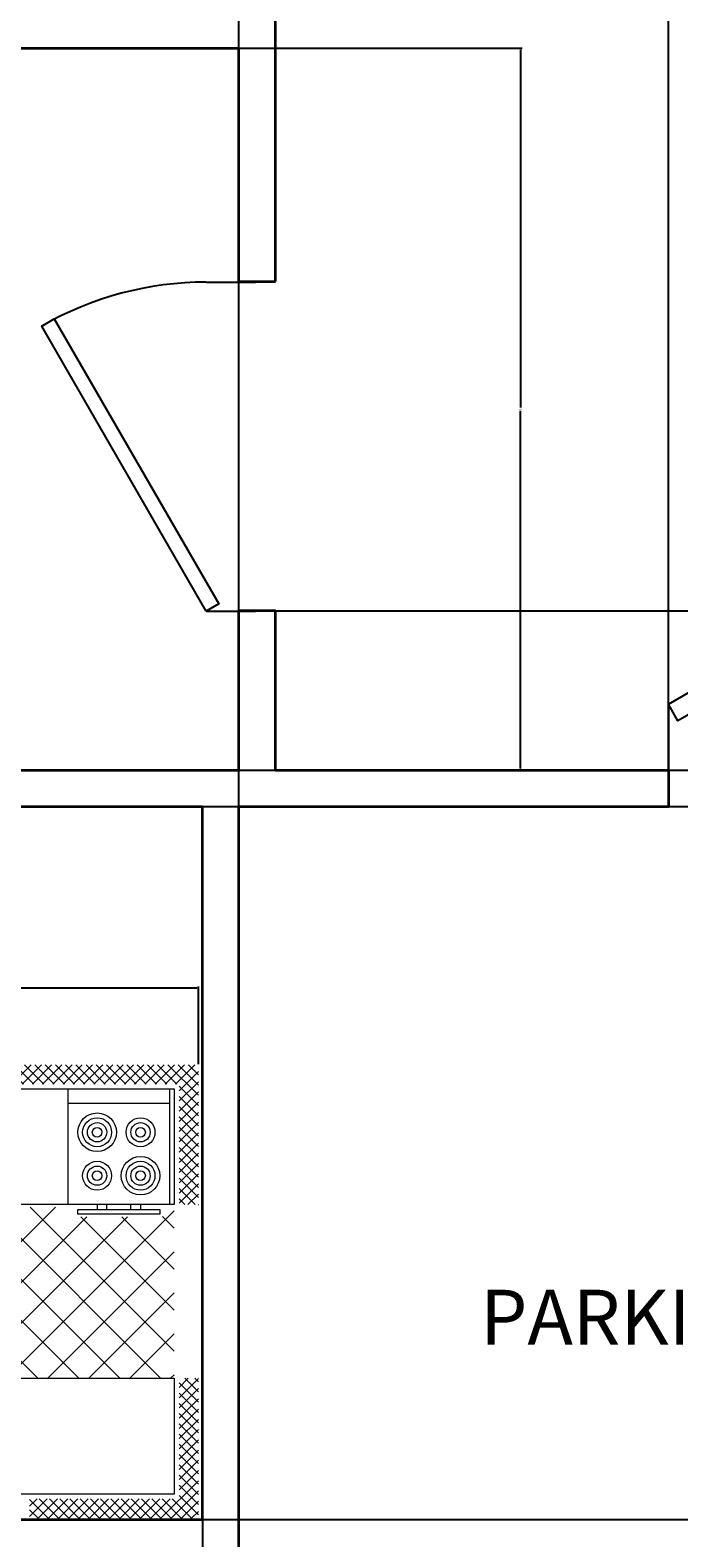
# Model space of a CAD drawing. Units: feet. Extents: x 3746 to 4170, y 1475 to 2148.
# Tile 3 of 5: x 3884 to 3955, y 1755 to 1920. Entities that reach past the tile are written whole.
import ezdxf

# ---------------------------------------------------------------- set-up
doc = ezdxf.new("R2010")
doc.units = ezdxf.units.FT
for name, color, linetype, lineweight in [('A-ANNO-DIMS', 2, 'Continuous', 18), ('A-AREA-IDEN', 7, 'Continuous', 25), ('A-FLOR-FIXT', 9, 'Continuous', 18), ('DOOR', 135, 'Continuous', 25), ('INWER WALL', 30, 'Continuous', 35)]:
    doc.layers.add(name, color=color, linetype=linetype, lineweight=lineweight)
doc.styles.get("Standard").update_dxf_attribs({"font": 'arial.ttf'})
doc.dimstyles.get("Standard").update_dxf_attribs({"dimtxt": 0.18, "dimasz": 0.18, "dimexe": 0.18, "dimexo": 0.0625, "dimgap": 0.09, "dimtad": 0, "dimtih": 1, "dimtoh": 1, "dimdec": 4, "dimzin": 0, "dimdsep": 46, "dimtxsty": 'Standard', "dimcen": 0.09, "dimadec": 0, "dimazin": 0, "dimtfac": 1, "dimtdec": 4, "dimtofl": 0, "dimtmove": 0, "dimatfit": 3, "dimfxl": 1, "dimtolj": 1, "dimtzin": 0, "dimarcsym": 0})

# ---------------------------------------------------------------- blocks, each defined once
blk = doc.blocks.new('*U2')
for p, q in [((0, 0), (0, -6)), ((40, 0), (40, -6))]:
    blk.add_line(p, q)
blk.add_lwpolyline([(0, 0), (34.64, 20), (35.52, 18.48), (0.87, -1.52)], close=True)
blk.add_arc((0, 0), 40, 0, 30)
blk = doc.blocks.new('Kitchen Layout - 7 x 8 ft')
for p, q in [((-5, 81.32), (2.68, 89)), ((-5, 83.44), (0.56, 89)), ((-5, 85.56), (-1.56, 89)), ((-5, 87.68), (-3.68, 89)), ((-1, 84.97), (-5, 88.97)), ((1.09, 85), (-2.91, 89)), ((3.21, 85), (-0.79, 89)), ((0.81, 85), (4.81, 89)), ((5.34, 85), (1.34, 89)), ((2.93, 85), (6.93, 89)), ((7.46, 85), (3.46, 89)), ((5.05, 85), (9.05, 89)), ((9.58, 85), (5.58, 89)), ((7.17, 85), (11.17, 89)), ((11.7, 85), (7.7, 89)), ((9.29, 85), (13.29, 89)), ((13.82, 85), (9.82, 89)), ((11.41, 85), (15.41, 89)), ((15.94, 85), (11.94, 89)), ((13.53, 85), (17.53, 89)), ((18.06, 85), (14.06, 89)), ((15.65, 85), (19.65, 89)), ((20.18, 85), (16.18, 89)), ((17.78, 85), (21.78, 89)), ((22.31, 85), (18.31, 89)), ((19.9, 85), (23.9, 89)), ((24.43, 85), (20.43, 89)), ((22.02, 85), (26.02, 89)), ((26.55, 85), (22.55, 89)), ((24.14, 85), (28.14, 89)), ((28.67, 85), (24.67, 89)), ((26.26, 85), (30.26, 89)), ((30.79, 85), (26.79, 89)), ((28.38, 85), (32.38, 89)), ((32.91, 85), (28.91, 89)), ((30.5, 85), (34.5, 89)), ((35.03, 85), (31.03, 89)), ((32.63, 85), (36.63, 89)), ((37.16, 85), (33.16, 89)), ((34.75, 85), (38.75, 89)), ((39.28, 85), (35.28, 89)), ((36.87, 85), (40.87, 89)), ((41.4, 85), (37.4, 89)), ((38.99, 85), (42.99, 89)), ((43.52, 85), (39.52, 89)), ((41.11, 85), (45.11, 89)), ((45.64, 85), (41.64, 89)), ((43.23, 85), (47.23, 89)), ((47.76, 85), (43.76, 89)), ((45.35, 85), (49.35, 89)), ((49.88, 85), (45.88, 89)), ((47.47, 85), (51.47, 89)), ((52, 85), (48, 89)), ((49.6, 85), (53.6, 89)), ((54.13, 85), (50.13, 89)), ((51.72, 85), (55.72, 89)), ((56.25, 85), (52.25, 89)), ((53.84, 85), (57.84, 89)), ((58.37, 85), (54.37, 89)), ((55.96, 85), (59.96, 89)), ((60.49, 85), (56.49, 89)), ((58.08, 85), (62.08, 89)), ((62.61, 85), (58.61, 89)), ((60.2, 85), (64.2, 89)), ((64.73, 85), (60.73, 89)), ((62.32, 85), (66.32, 89)), ((66.85, 85), (62.85, 89)), ((64.45, 85), (68.45, 89)), ((68.97, 85), (64.97, 89)), ((66.57, 85), (70.57, 89)), ((71.1, 85), (67.1, 89)), ((68.69, 85), (72.69, 89)), ((73.22, 85), (69.22, 89)), ((70.81, 85), (74.81, 89)), ((75.34, 85), (71.34, 89)), ((72.93, 85), (76.93, 89)), ((77.46, 85), (73.46, 89)), ((75.05, 85), (79.05, 89)), ((79.58, 85), (75.58, 89)), ((77.17, 85), (81.17, 89)), ((81.7, 85), (77.7, 89)), ((79.29, 85), (83.29, 89)), ((83.82, 85), (79.82, 89)), ((81.42, 85), (85.42, 89)), ((85.95, 85), (81.95, 89)), ((83.54, 85), (87.54, 89)), ((88.07, 85), (84.07, 89)), ((85.66, 85), (89.66, 89)), ((90.19, 85), (86.19, 89)), ((87.78, 85), (91.78, 89)), ((92.31, 85), (88.31, 89)), ((89.9, 85), (93.9, 89)), ((94.43, 85), (90.43, 89)), ((92.02, 85), (96.02, 89)), ((96.55, 85), (92.55, 89)), ((94.14, 85), (98.14, 89)), ((101, 82.67), (94.67, 89)), ((96.27, 85), (100.27, 89)), ((101, 84.79), (96.79, 89)), ((97, 83.61), (101, 87.61)), ((101, 86.92), (98.92, 89)), ((-1, 82.85), (-5, 86.85)), ((-1, 80.73), (-5, 84.73)), ((97, 81.49), (101, 85.49)), ((101, 80.55), (97, 84.55)), ((-5, 79.19), (-1, 83.19)), ((-1, 78.61), (-5, 82.61)), ((34, 84), (96, 84)), ((34, 60), (34, 84)), ((96, 84), (96, 60)), ((97, 79.37), (101, 83.37)), ((101, 78.43), (97, 82.43)), ((-5, 77.07), (-1, 81.07)), ((-1, 76.49), (-5, 80.49)), ((-5, 74.95), (-1, 78.95)), ((-1, 74.36), (-5, 78.36)), ((74, 81), (95, 81)), ((97, 77.25), (101, 81.25)), ((101, 76.31), (97, 80.31)), ((97, 75.13), (101, 79.13)), ((101, 74.19), (97, 78.19)), ((-5, 72.83), (-1, 76.83)), ((-1, 72.24), (-5, 76.24)), ((97, 73.01), (101, 77.01)), ((101, 72.07), (97, 76.07)), ((-5, 70.71), (-1, 74.71)), ((-1, 70.12), (-5, 74.12)), ((-5, 68.59), (-1, 72.59)), ((-1, 68), (-5, 72)), ((97, 70.89), (101, 74.89)), ((101, 69.95), (97, 73.95)), ((97, 68.76), (101, 72.76)), ((-5, 66.47), (-1, 70.47)), ((-1, 65.88), (-5, 69.88)), ((101, 67.82), (97, 71.82)), ((97, 66.64), (101, 70.64)), ((101, 65.7), (97, 69.7)), ((-5, 64.35), (-1, 68.35)), ((-1, 63.76), (-5, 67.76)), ((-5, 62.22), (-1, 66.22)), ((-1, 61.64), (-5, 65.64)), ((97, 64.52), (101, 68.52)), ((101, 63.58), (97, 67.58)), ((97, 62.4), (101, 66.4)), ((-5, 60.1), (-1, 64.1)), ((-1, 59.52), (-5, 63.52)), ((101, 61.46), (97, 65.46)), ((97, 60.28), (101, 64.28)), ((100.34, 60), (97, 63.34)), ((-5, 57.98), (-1, 61.98)), ((-1, 57.39), (-5, 61.39)), ((-4.86, 56), (-1, 59.86)), ((10.4, 24), (45.9, 59.5)), ((18.88, 24), (54.38, 59.5)), ((27.37, 24), (62.87, 59.5)), ((33.03, 55.11), (37.41, 59.5)), ((96, 60), (34, 60)), ((35.85, 24), (71.35, 59.5)), ((76.2, 24), (40.7, 59.5)), ((84.68, 24), (49.18, 59.5)), ((93.17, 24), (57.67, 59.5)), ((96, 29.65), (66.15, 59.5)), ((80, 60), (80, 59)), ((82, 59), (82, 60)), ((87, 59), (87, 60)), ((89, 60), (89, 59)), ((98.22, 60), (97, 61.22)), ((98.84, 60), (101, 62.16)), ((100.96, 60), (101, 60.04)), ((-1.73, 56), (-5, 59.27)), ((-3.85, 56), (-5, 57.15)), ((-2.74, 56), (-1, 57.74)), ((0, 57), (33, 57)), ((67.71, 24), (33.68, 58.04)), ((44.34, 24), (77.84, 57.5)), ((52.82, 24), (86.32, 57.5)), ((61.31, 24), (96, 58.69)), ((96, 38.14), (76.64, 57.5)), ((96, 46.63), (85.13, 57.5)), ((96, 55.11), (93.57, 57.54)), ((0, 30.57), (24.43, 55)), ((0, 39.06), (15.94, 55)), ((0, 47.54), (7.46, 55)), ((1.91, 24), (32.91, 55)), ((33.77, 24), (2.77, 55)), ((42.26, 24), (11.26, 55)), ((50.74, 24), (19.74, 55)), ((59.23, 24), (28.23, 55)), ((31, 55), (31, 56)), ((32, 55), (31, 55)), ((32, 56), (32, 55)), ((69.79, 24), (96, 50.21)), ((25.29, 24), (0, 49.29)), ((16.8, 24), (0, 40.8)), ((78.28, 24), (96, 41.72)), ((8.32, 24), (0, 32.32)), ((86.76, 24), (96, 33.24)), ((-5, 21.92), (-2.92, 24)), ((-5, 19.8), (-1, 23.8)), ((-1, 19.21), (-5, 23.21)), ((-1, 21.33), (-3.67, 24)), ((-1, 23.45), (-1.55, 24)), ((0, 24), (96, 24)), ((0, 0), (0, 24)), ((95.25, 24), (96, 24.75)), ((96, 24), (96, 0)), ((97, 22.1), (98.9, 24)), ((97, 19.97), (101, 23.97)), ((101, 19.03), (97, 23.03)), ((101, 21.16), (98.16, 24)), ((101, 23.28), (100.28, 24)), ((-5, 17.68), (-1, 21.68)), ((-1, 17.09), (-5, 21.09)), ((-5, 15.55), (-1, 19.55)), ((-1, 14.97), (-5, 18.97)), ((97, 17.85), (101, 21.85)), ((101, 16.91), (97, 20.91)), ((97, 15.73), (101, 19.73)), ((101, 14.79), (97, 18.79)), ((-5, 13.43), (-1, 17.43)), ((-1, 12.85), (-5, 16.85)), ((47.25, 6.5), (47.25, 18.5)), ((48.75, 18.5), (48.75, 6.5)), ((97, 13.61), (101, 17.61)), ((101, 12.67), (97, 16.67)), ((-5, 11.31), (-1, 15.31)), ((-1, 10.73), (-5, 14.73)), ((-5, 9.19), (-1, 13.19)), ((-1, 8.6), (-5, 12.6)), ((97, 11.49), (101, 15.49)), ((101, 10.55), (97, 14.55)), ((97, 9.37), (101, 13.37)), ((-5, 7.07), (-1, 11.07)), ((-1, 6.48), (-5, 10.48)), ((101, 8.43), (97, 12.43)), ((97, 7.25), (101, 11.25)), ((101, 6.31), (97, 10.31)), ((-5, 4.95), (-1, 8.95)), ((-1, 4.36), (-5, 8.36)), ((-5, 2.83), (-1, 6.83)), ((97, 5.12), (101, 9.12)), ((101, 4.18), (97, 8.18)), ((97, 3), (101, 7)), ((-1, 2.24), (-5, 6.24)), ((-5, 0.71), (-1, 4.71)), ((-1, 0.12), (-5, 4.12)), ((64, 4), (32, 4)), ((101, 2.06), (97, 6.06)), ((97, 0.88), (101, 4.88)), ((101, -0.06), (97, 3.94)), ((-5, -1.42), (-1, 2.58)), ((2, -5), (-5, 2)), ((-5, -3.54), (-1, 0.46)), ((96, 0), (0, 0)), ((93.24, -5), (101, 2.76)), ((95.36, -5), (101, 0.64)), ((101, -2.18), (97, 1.82)), ((-0.12, -5), (-5, -0.12)), ((-2.25, -5), (-5, -2.25)), ((-4.34, -5), (-0.34, -1)), ((-2.22, -5), (1.78, -1)), ((-0.1, -5), (3.9, -1)), ((4.12, -5), (0.12, -1)), ((2.02, -5), (6.02, -1)), ((6.24, -5), (2.24, -1)), ((4.14, -5), (8.14, -1)), ((8.36, -5), (4.36, -1)), ((6.27, -5), (10.27, -1)), ((10.48, -5), (6.48, -1)), ((8.39, -5), (12.39, -1)), ((12.6, -5), (8.6, -1)), ((10.51, -5), (14.51, -1)), ((14.73, -5), (10.73, -1)), ((12.63, -5), (16.63, -1)), ((16.85, -5), (12.85, -1)), ((14.75, -5), (18.75, -1)), ((18.97, -5), (14.97, -1)), ((16.87, -5), (20.87, -1)), ((21.09, -5), (17.09, -1)), ((18.99, -5), (22.99, -1)), ((23.21, -5), (19.21, -1)), ((21.11, -5), (25.11, -1)), ((25.33, -5), (21.33, -1)), ((23.24, -5), (27.24, -1)), ((27.45, -5), (23.45, -1)), ((25.36, -5), (29.36, -1)), ((29.57, -5), (25.57, -1)), ((27.48, -5), (30, -2.48)), ((30, -3.3), (27.7, -1)), ((30, -1.18), (29.82, -1)), ((66, -2.54), (67.54, -1)), ((66, -4.66), (69.66, -1)), ((69.88, -5), (66, -1.12)), ((67.78, -5), (71.78, -1)), ((72, -5), (68, -1)), ((69.9, -5), (73.9, -1)), ((74.12, -5), (70.12, -1)), ((72.03, -5), (76.03, -1)), ((76.24, -5), (72.24, -1)), ((74.15, -5), (78.15, -1)), ((78.36, -5), (74.36, -1)), ((76.27, -5), (80.27, -1)), ((80.49, -5), (76.49, -1)), ((78.39, -5), (82.39, -1)), ((82.61, -5), (78.61, -1)), ((80.51, -5), (84.51, -1)), ((84.73, -5), (80.73, -1)), ((82.63, -5), (86.63, -1)), ((86.85, -5), (82.85, -1)), ((84.75, -5), (88.75, -1)), ((88.97, -5), (84.97, -1)), ((86.88, -5), (90.88, -1)), ((91.09, -5), (87.09, -1)), ((89, -5), (93, -1)), ((93.21, -5), (89.21, -1)), ((91.12, -5), (95.12, -1)), ((95.34, -5), (91.34, -1)), ((97.46, -5), (93.46, -1)), ((99.58, -5), (95.58, -1)), ((101, -4.3), (97, -0.3)), ((97.48, -5), (101, -1.48)), ((-4.37, -5), (-5, -4.37)), ((29.6, -5), (30, -4.6)), ((67.76, -5), (66, -3.24)), ((99.6, -5), (101, -3.6))]:
    blk.add_line(p, q)
for points in [[(0, 56), (0, 84), (33, 84), (33, 56)], [(74, 60), (74, 84), (95, 84), (95, 60)], [(76, 58), (76, 59), (93, 59), (93, 58)]]:
    blk.add_lwpolyline(points, close=True)
for points in [[(32, 1.5), (32, 19.5)], [(33.5, 21), (62.5, 21)], [(34.5, 19.5), (46.25, 19.5)], [(49.75, 19.5), (61.5, 19.5)], [(64, 19.5), (64, 1.5)], [(33.5, 6.5), (33.5, 18.5)], [(62.5, 18.5), (62.5, 6.5)], [(46.25, 5.5), (34.5, 5.5)], [(61.5, 5.5), (49.75, 5.5)], [(62.5, 0), (33.5, 0)]]:
    blk.add_lwpolyline(points)
for centre, radius in [((80, 75), 4), ((80, 75), 3), ((80, 75), 2), ((80, 75), 1), ((89, 75), 3), ((89, 75), 2), ((89, 75), 1), ((80, 66), 3), ((89, 66), 4), ((89, 66), 3), ((80, 66), 2), ((80, 66), 1), ((89, 66), 2), ((89, 66), 1), ((40.5, 12.5), 1), ((40.5, 12.5), 0.5), ((55.5, 12.5), 1), ((55.5, 12.5), 0.5)]:
    blk.add_circle(centre, radius)
for centre, radius, start, end in [((33.5, 19.5), 1.5, 90, 180), ((34.5, 18.5), 1, 90, 180), ((46.25, 18.5), 1, 0, 90), ((49.75, 18.5), 1, 90, 180), ((61.5, 18.5), 1, 0, 90), ((62.5, 19.5), 1.5, 0, 90), ((34.5, 6.5), 1, 180, 270), ((46.25, 6.5), 1, 270, 0), ((49.75, 6.5), 1, 180, 270), ((61.5, 6.5), 1, 270, 0), ((33.5, 1.5), 1.5, 180, 270), ((62.5, 1.5), 1.5, 270, 0)]:
    blk.add_arc(centre, radius, start, end)
blk = doc.blocks.new('*D49')
at = {"layer": 'A-ANNO-DIMS', "color": 0, "lineweight": -2, "transparency": 16777216}
for p, q in [((3846.04, 1807.21), (3846.04, 1815.72)), ((3846.22, 1815.54), (3872.88, 1815.54)), ((3901.8, 1815.54), (3875.14, 1815.54)), ((3901.98, 1807.21), (3901.98, 1815.72))]:
    blk.add_line(p, q, dxfattribs=at)
at = {"layer": 'A-ANNO-DIMS', "color": 0, "transparency": 16777216}
for points in [[(3846.22, 1815.57), (3846.22, 1815.51), (3846.04, 1815.54)], [(3901.8, 1815.57), (3901.8, 1815.51), (3901.98, 1815.54)]]:
    blk.add_solid(points, dxfattribs=at)
at = {"layer": 'Defpoints', "color": 0, "transparency": 16777216}
for p in [(3901.98, 1815.54), (3846.04, 1807.14), (3901.98, 1807.14)]:
    blk.add_point(p, dxfattribs=at)
at = {"layer": 'A-ANNO-DIMS', "color": 0, "transparency": 16777216, "insert": (3874.01, 1815.54), "char_height": 0.18, "attachment_point": 5}
blk.add_mtext('\\A1;KITCHEN UNIT 56', dxfattribs=at)
blk = doc.blocks.new('*D65')
at = {"layer": 'A-ANNO-DIMS', "color": 0, "lineweight": -2, "transparency": 16777216}
for p, q in [((3906.49, 1918.38), (3937.41, 1918.38)), ((3937.23, 1918.2), (3937.23, 1879.06)), ((3937.23, 1839.56), (3937.23, 1878.7)), ((3906.49, 1839.38), (3937.41, 1839.38))]:
    blk.add_line(p, q, dxfattribs=at)
at = {"layer": 'A-ANNO-DIMS', "color": 0, "transparency": 16777216}
for points in [[(3937.2, 1918.2), (3937.26, 1918.2), (3937.23, 1918.38)], [(3937.2, 1839.56), (3937.26, 1839.56), (3937.23, 1839.38)]]:
    blk.add_solid(points, dxfattribs=at)
at = {"layer": 'Defpoints', "color": 0, "transparency": 16777216}
for p in [(3906.43, 1918.38), (3906.43, 1839.38), (3937.23, 1839.38)]:
    blk.add_point(p, dxfattribs=at)
at = {"layer": 'A-ANNO-DIMS', "color": 0, "transparency": 16777216, "insert": (3937.23, 1878.88), "char_height": 0.18, "attachment_point": 5}
blk.add_mtext('\\A1;79', dxfattribs=at)
blk = doc.blocks.new('*D66')
at = {"layer": 'A-ANNO-DIMS', "color": 0, "lineweight": -2, "transparency": 16777216}
for p, q in [((3786.43, 1918.45), (3786.43, 2147.69)), ((3786.61, 2147.51), (3846.15, 2147.51)), ((3906.25, 2147.51), (3846.71, 2147.51)), ((3906.43, 1918.45), (3906.43, 2147.69))]:
    blk.add_line(p, q, dxfattribs=at)
at = {"layer": 'A-ANNO-DIMS', "color": 0, "transparency": 16777216}
for points in [[(3786.61, 2147.54), (3786.61, 2147.48), (3786.43, 2147.51)], [(3906.25, 2147.54), (3906.25, 2147.48), (3906.43, 2147.51)]]:
    blk.add_solid(points, dxfattribs=at)
at = {"layer": 'Defpoints', "color": 0, "transparency": 16777216}
for p in [(3906.43, 2147.51), (3786.43, 1918.38), (3906.43, 1918.38)]:
    blk.add_point(p, dxfattribs=at)
at = {"layer": 'A-ANNO-DIMS', "color": 0, "transparency": 16777216, "insert": (3846.43, 2147.51), "char_height": 0.18, "attachment_point": 5}
blk.add_mtext('\\A1;120', dxfattribs=at)
blk = doc.blocks.new('*D67')
at = {"layer": 'A-ANNO-DIMS', "color": 0, "lineweight": -2, "transparency": 16777216}
for p, q in [((3902.49, 1835.38), (4169.74, 1835.38)), ((4169.56, 1835.2), (4169.56, 1796.56)), ((4169.56, 1757.56), (4169.56, 1796.2)), ((3902.49, 1757.38), (4169.74, 1757.38))]:
    blk.add_line(p, q, dxfattribs=at)
at = {"layer": 'A-ANNO-DIMS', "color": 0, "transparency": 16777216}
for points in [[(4169.53, 1835.2), (4169.59, 1835.2), (4169.56, 1835.38)], [(4169.53, 1757.56), (4169.59, 1757.56), (4169.56, 1757.38)]]:
    blk.add_solid(points, dxfattribs=at)
at = {"layer": 'Defpoints', "color": 0, "transparency": 16777216}
for p in [(3902.43, 1835.38), (3902.43, 1757.38), (4169.56, 1757.38)]:
    blk.add_point(p, dxfattribs=at)
at = {"layer": 'A-ANNO-DIMS', "color": 0, "transparency": 16777216, "insert": (4169.56, 1796.38), "char_height": 0.18, "attachment_point": 5}
blk.add_mtext('\\A1;78', dxfattribs=at)
blk = doc.blocks.new('*D68')
at = {"layer": 'A-ANNO-DIMS', "color": 0, "lineweight": -2, "transparency": 16777216}
for p, q in [((3786.43, 1757.32), (3786.43, 1474.8)), ((3902.43, 1757.32), (3902.43, 1474.8)), ((3786.61, 1474.98), (3844.15, 1474.98)), ((3902.25, 1474.98), (3844.71, 1474.98))]:
    blk.add_line(p, q, dxfattribs=at)
at = {"layer": 'A-ANNO-DIMS', "color": 0, "transparency": 16777216}
for points in [[(3786.61, 1475.01), (3786.61, 1474.95), (3786.43, 1474.98)], [(3902.25, 1475.01), (3902.25, 1474.95), (3902.43, 1474.98)]]:
    blk.add_solid(points, dxfattribs=at)
at = {"layer": 'Defpoints', "color": 0, "transparency": 16777216}
for p in [(3786.43, 1757.38), (3902.43, 1757.38), (3902.43, 1474.98)]:
    blk.add_point(p, dxfattribs=at)
at = {"layer": 'A-ANNO-DIMS', "color": 0, "transparency": 16777216, "insert": (3844.43, 1474.98), "char_height": 0.18, "attachment_point": 5}
blk.add_mtext('\\A1;116', dxfattribs=at)
blk = doc.blocks.new('*D77')
at = {"layer": 'A-ANNO-DIMS', "color": 0, "lineweight": -2, "transparency": 16777216}
for p, q in [((3953.43, 1839.45), (3953.43, 2147.69)), ((3953.61, 2147.51), (3977.21, 2147.51)), ((4001.25, 2147.51), (3977.65, 2147.51)), ((4001.43, 1839.45), (4001.43, 2147.69))]:
    blk.add_line(p, q, dxfattribs=at)
at = {"layer": 'A-ANNO-DIMS', "color": 0, "transparency": 16777216}
for points in [[(3953.61, 2147.54), (3953.61, 2147.48), (3953.43, 2147.51)], [(4001.25, 2147.54), (4001.25, 2147.48), (4001.43, 2147.51)]]:
    blk.add_solid(points, dxfattribs=at)
at = {"layer": 'Defpoints', "color": 0, "transparency": 16777216}
for p in [(4001.43, 2147.51), (3953.43, 1839.38), (4001.43, 1839.38)]:
    blk.add_point(p, dxfattribs=at)
at = {"layer": 'A-ANNO-DIMS', "color": 0, "transparency": 16777216, "insert": (3977.43, 2147.51), "char_height": 0.18, "attachment_point": 5}
blk.add_mtext('\\A1;48', dxfattribs=at)
blk = doc.blocks.new('*D78')
at = {"layer": 'A-ANNO-DIMS', "color": 0, "lineweight": -2, "transparency": 16777216}
for p, q in [((3906.43, 1835.45), (3906.43, 2147.69)), ((3906.61, 2147.51), (3929.71, 2147.51)), ((3953.25, 2147.51), (3930.15, 2147.51)), ((3953.43, 1835.45), (3953.43, 2147.69))]:
    blk.add_line(p, q, dxfattribs=at)
at = {"layer": 'A-ANNO-DIMS', "color": 0, "transparency": 16777216}
for points in [[(3906.61, 2147.54), (3906.61, 2147.48), (3906.43, 2147.51)], [(3953.25, 2147.54), (3953.25, 2147.48), (3953.43, 2147.51)]]:
    blk.add_solid(points, dxfattribs=at)
at = {"layer": 'Defpoints', "color": 0, "transparency": 16777216}
for p in [(3953.43, 2147.51), (3906.43, 1835.38), (3953.43, 1835.38)]:
    blk.add_point(p, dxfattribs=at)
at = {"layer": 'A-ANNO-DIMS', "color": 0, "transparency": 16777216, "insert": (3929.93, 2147.51), "char_height": 0.18, "attachment_point": 5}
blk.add_mtext('\\A1;47', dxfattribs=at)
blk = doc.blocks.new('*D89')
at = {"layer": 'A-ANNO-DIMS', "color": 0, "lineweight": -2, "transparency": 16777216}
for p, q in [((3906.49, 1856.82), (4169.74, 1856.82)), ((4169.56, 1856.64), (4169.56, 1848.28)), ((4169.56, 1839.56), (4169.56, 1847.92)), ((3906.49, 1839.38), (4169.74, 1839.38))]:
    blk.add_line(p, q, dxfattribs=at)
at = {"layer": 'A-ANNO-DIMS', "color": 0, "transparency": 16777216}
for points in [[(4169.53, 1856.64), (4169.59, 1856.64), (4169.56, 1856.82)], [(4169.53, 1839.56), (4169.59, 1839.56), (4169.56, 1839.38)]]:
    blk.add_solid(points, dxfattribs=at)
at = {"layer": 'Defpoints', "color": 0, "transparency": 16777216}
for p in [(3906.43, 1856.82), (4169.56, 1856.82), (3906.43, 1839.38)]:
    blk.add_point(p, dxfattribs=at)
at = {"layer": 'A-ANNO-DIMS', "color": 0, "transparency": 16777216, "insert": (4169.56, 1848.1), "char_height": 0.18, "attachment_point": 5}
blk.add_mtext('\\A1;17.442', dxfattribs=at)

msp = doc.modelspace()

# ---------------------------------------------------------------- linework, layer by layer
at = {"layer": 'INWER WALL'}
for p, q in [((3910.4289, 1892.8248), (3910.4289, 1922.3828)), ((3786.4289, 1918.3828), (3906.4289, 1918.3828)), ((3906.4289, 1892.8248), (3906.4289, 1918.3828)), ((3906.4289, 1892.8248), (3906.4289, 1918.3828)), ((3906.4289, 1892.8248), (3910.4289, 1892.8248)), ((3906.4289, 1839.3828), (3906.4289, 1856.8248)), ((3906.4289, 1856.8248), (3910.4289, 1856.8248)), ((3906.4289, 1839.3828), (3906.4289, 1856.8248)), ((3910.4289, 1839.3828), (3910.4289, 1856.8248)), ((3838.6077, 1839.3828), (3906.4289, 1839.3828)), ((3910.4289, 1839.3828), (3953.4289, 1839.3828)), ((3953.4289, 1839.3828), (3953.4289, 1835.3828)), ((3838.6077, 1835.3828), (3902.4289, 1835.3828)), ((3902.4289, 1757.3828), (3902.4289, 1835.3828)), ((3906.4289, 1753.3828), (3906.4289, 1835.3828)), ((3906.4289, 1835.3828), (3953.4289, 1835.3828)), ((3786.4289, 1757.3828), (3902.4289, 1757.3828))]:
    msp.add_line(p, q, dxfattribs=at)

# ---------------------------------------------------------------- block references
at = {"layer": 'A-FLOR-FIXT', "xscale": 0.5277695624753019, "yscale": 0.5277695624753019, "zscale": 0.5277695624753019}
msp.add_blockref('Kitchen Layout - 7 x 8 ft', (3848.6802, 1760.1735), dxfattribs=at)
at = {"layer": 'DOOR', "xscale": 0.9000000000000054, "yscale": 0.9000000000000054, "zscale": 0.9000000000000054, "rotation": 90}
msp.add_blockref('*U2', (3902.8507, 1856.7718), dxfattribs=at)
at = {"layer": 'DOOR', "xscale": 1.200000000000002, "yscale": 1.200000000000002, "zscale": 1.200000000000002}
msp.add_blockref('*U2', (3953.4289, 1846.5828), dxfattribs=at)

# ---------------------------------------------------------------- texts
at = {"layer": 'A-AREA-IDEN', "insert": (3932.8141, 1782.5296), "char_height": 6, "attachment_point": 1}
msp.add_mtext_dynamic_manual_height_columns('PARKING', width=45.721785, gutter_width=12.5, heights=[0], dxfattribs=at)

# ---------------------------------------------------------------- dimensions: what is measured, and where the dimension line sits
at = {"layer": 'A-ANNO-DIMS'}
for base, p1, p2, picture, middle in [((3906.4289, 2147.5109), (3786.4289, 1918.3828), (3906.4289, 1918.3828), '*D66', (3846.4289, 2147.5109)), ((3953.4289, 2147.5109), (3906.4289, 1835.3828), (3953.4289, 1835.3828), '*D78', (3929.9289, 2147.5109)), ((4001.4289, 2147.5109), (3953.4289, 1839.3828), (4001.4289, 1839.3828), '*D77', (3977.4289, 2147.5109)), ((3902.4289, 1474.98), (3786.4289, 1757.3828), (3902.4289, 1757.3828), '*D68', (3844.4289, 1474.98))]:
    dim = msp.add_linear_dim(base=base, p1=p1, p2=p2, dimstyle='Standard', override={"dimdec": 0, "dimlfac": 1, "dimrnd": 0, "dimzin": 0, "dimdsep": 46, "dimlunit": 2}, dxfattribs=at)
    dim.commit()
    dim.dimension.update_dxf_attribs({"geometry": picture, "text_midpoint": middle})
for base, p1, p2, angle, override, picture, middle in [((3937.2289, 1839.3828), (3906.4289, 1918.3828), (3906.4289, 1839.3828), 270, {"dimdec": 0, "dimlfac": 1, "dimrnd": 0, "dimzin": 0, "dimdsep": 46, "dimlunit": 2}, '*D65', (3937.2289, 1878.8828)), ((4169.5569, 1856.8248), (3906.4289, 1839.3828), (3906.4289, 1856.8248), 90, {"dimdec": 3, "dimlfac": 1, "dimrnd": 0, "dimzin": 0, "dimdsep": 46, "dimlunit": 2}, '*D89', (4169.5569, 1848.1038)), ((4169.5569, 1757.3828), (3902.4289, 1835.3828), (3902.4289, 1757.3828), 90, {"dimdec": 0, "dimlfac": 1, "dimrnd": 0, "dimzin": 0, "dimdsep": 46, "dimlunit": 2}, '*D67', (4169.5569, 1796.3828))]:
    dim = msp.add_linear_dim(base=base, p1=p1, p2=p2, angle=angle, dimstyle='Standard', override=override, dxfattribs=at)
    dim.commit()
    dim.dimension.update_dxf_attribs({"geometry": picture, "text_midpoint": middle})
dim = msp.add_linear_dim(base=(3901.985, 1815.5365), p1=(3846.0414, 1807.145), p2=(3901.985, 1807.145), text='KITCHEN UNIT <>', dimstyle='Standard', override={"dimdec": 0, "dimlfac": 1, "dimrnd": 0, "dimzin": 0, "dimdsep": 46, "dimlunit": 2}, dxfattribs=at)
dim.commit()
dim.dimension.update_dxf_attribs({"geometry": '*D49', "text_midpoint": (3874.0132, 1815.5365)})

doc.saveas('drawing.dxf')
